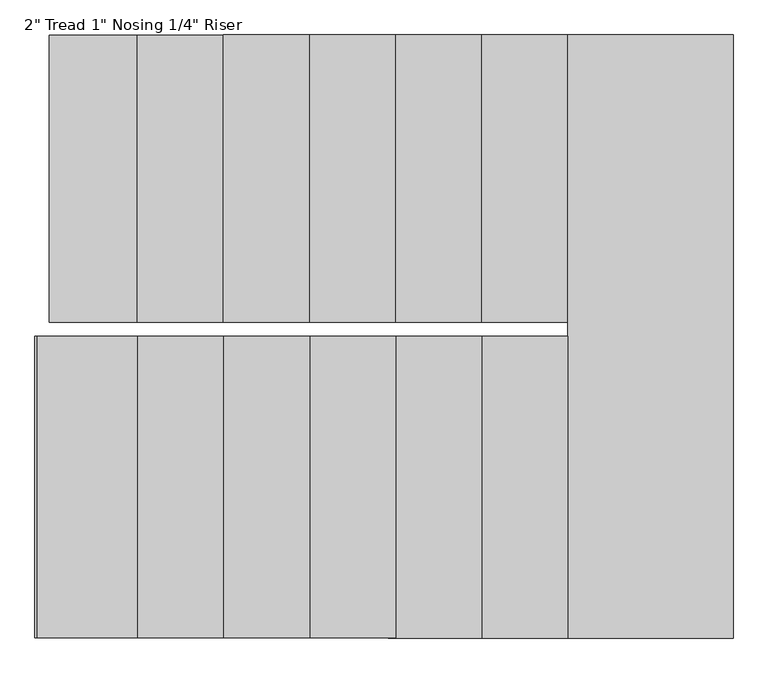
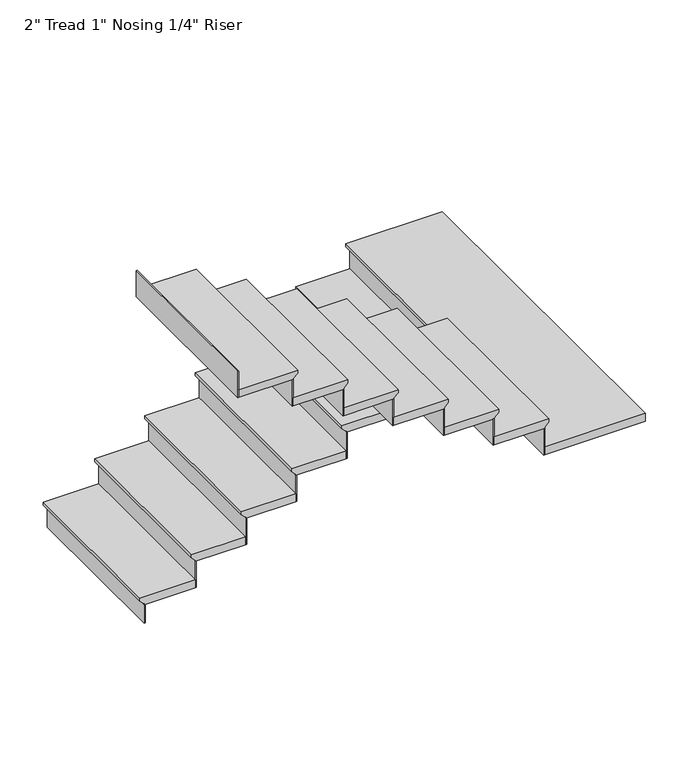
"""IFC4 building model written with IfcOpenShell, lengths in millimetres: stair flight geometry."""

from ifc_helpers import new_model, si_unit, origin, place, context, project, spatial, faceted_brep, source, transform, mapped, element, save


def stair_flight_57dbdc02(model_context):
    return source(origin(), model_context, "Body", "Brep", [
        faceted_brep([(-1167.6638307, -167.7482799, 12951.8833333), (-1167.6638307, -167.7482799, 12970.9333333), (-1167.6638307, 848.2517201, 12970.9333333), (-1167.6638307, 848.2517201, 12951.8833333), (-1142.2638307, -167.7482799, 12926.4833333), (-1142.2638307, 848.2517201, 12926.4833333), (-831.1138307, -167.7482799, 12970.9333333), (-831.1138307, 848.2517201, 12970.9333333), (-1142.2638307, 848.2517201, 12920.1333333), (-831.1138307, 848.2517201, 12920.1333333), (-831.1138307, -167.7482799, 12920.1333333), (-1142.2638307, -167.7482799, 12920.1333333)], [[[0, 1, 2, 3]], [[4, 0, 3, 5]], [[2, 1, 6, 7]], [[8, 9, 10, 11]], [[2, 7, 9, 8, 5, 3]], [[8, 11, 4, 5]], [[6, 1, 0, 4, 11, 10]], [[7, 6, 10, 9]]]),
        faceted_brep([(-1142.2638307, -167.7482799, 12920.1333333), (-1142.2638307, -167.7482799, 12801.6), (-1135.9138307, -167.7482799, 12801.6), (-1135.9138307, -167.7482799, 12920.1333333), (-1142.2638307, 848.2517201, 12920.1333333), (-1135.9138307, 848.2517201, 12920.1333333), (-1135.9138307, 848.2517201, 12801.6), (-1142.2638307, 848.2517201, 12801.6)], [[[0, 1, 2, 3]], [[4, 5, 6, 7]], [[1, 0, 4, 7]], [[2, 1, 7, 6]], [[3, 2, 6, 5]], [[0, 3, 5, 4]]]),
        faceted_brep([(-831.1138307, -167.7482799, 13089.4666667), (-831.1138307, -167.7482799, 12920.1333333), (-824.7638307, -167.7482799, 12920.1333333), (-824.7638307, -167.7482799, 13089.4666667), (-831.1138307, 848.2517201, 13089.4666667), (-824.7638307, 848.2517201, 13089.4666667), (-824.7638307, 848.2517201, 12920.1333333), (-831.1138307, 848.2517201, 12920.1333333)], [[[0, 1, 2, 3]], [[4, 5, 6, 7]], [[1, 0, 4, 7]], [[2, 1, 7, 6]], [[3, 2, 6, 5]], [[0, 3, 5, 4]]]),
        faceted_brep([(-856.5138307, 848.2517201, 13140.2666667), (-856.5138307, -167.7482799, 13140.2666667), (-526.3138307, -167.7482799, 13140.2666667), (-526.3138307, 848.2517201, 13140.2666667), (-831.1138307, 848.2517201, 13089.4666667), (-526.3138307, 848.2517201, 13089.4666667), (-526.3138307, -167.7482799, 13089.4666667), (-831.1138307, -167.7482799, 13089.4666667), (-831.1138307, 848.2517201, 13095.8166667), (-856.5138307, 848.2517201, 13121.2166667), (-831.1138307, -167.7482799, 13095.8166667), (-856.5138307, -167.7482799, 13121.2166667)], [[[0, 1, 2, 3]], [[4, 5, 6, 7]], [[0, 3, 5, 4, 8, 9]], [[4, 7, 10, 8]], [[2, 1, 11, 10, 7, 6]], [[3, 2, 6, 5]], [[11, 1, 0, 9]], [[10, 11, 9, 8]]]),
        faceted_brep([(-526.3138307, -167.7482799, 13258.8), (-526.3138307, -167.7482799, 13089.4666667), (-519.9638307, -167.7482799, 13089.4666667), (-519.9638307, -167.7482799, 13258.8), (-526.3138307, 848.2517201, 13258.8), (-519.9638307, 848.2517201, 13258.8), (-519.9638307, 848.2517201, 13089.4666667), (-526.3138307, 848.2517201, 13089.4666667)], [[[0, 1, 2, 3]], [[4, 5, 6, 7]], [[1, 0, 4, 7]], [[2, 1, 7, 6]], [[3, 2, 6, 5]], [[0, 3, 5, 4]]]),
        faceted_brep([(-551.7138307, 848.2517201, 13309.6), (-551.7138307, -167.7482799, 13309.6), (-221.5138307, -167.7482799, 13309.6), (-221.5138307, 848.2517201, 13309.6), (-526.3138307, 848.2517201, 13258.8), (-221.5138307, 848.2517201, 13258.8), (-221.5138307, -167.7482799, 13258.8), (-526.3138307, -167.7482799, 13258.8), (-526.3138307, 848.2517201, 13265.15), (-551.7138307, 848.2517201, 13290.55), (-526.3138307, -167.7482799, 13265.15), (-551.7138307, -167.7482799, 13290.55)], [[[0, 1, 2, 3]], [[4, 5, 6, 7]], [[0, 3, 5, 4, 8, 9]], [[4, 7, 10, 8]], [[2, 1, 11, 10, 7, 6]], [[3, 2, 6, 5]], [[11, 1, 0, 9]], [[10, 11, 9, 8]]]),
        faceted_brep([(-221.5138307, -167.7482799, 13428.1333333), (-221.5138307, -167.7482799, 13258.8), (-215.1638307, -167.7482799, 13258.8), (-215.1638307, -167.7482799, 13428.1333333), (-221.5138307, 848.2517201, 13428.1333333), (-215.1638307, 848.2517201, 13428.1333333), (-215.1638307, 848.2517201, 13258.8), (-221.5138307, 848.2517201, 13258.8)], [[[0, 1, 2, 3]], [[4, 5, 6, 7]], [[1, 0, 4, 7]], [[2, 1, 7, 6]], [[3, 2, 6, 5]], [[0, 3, 5, 4]]]),
        faceted_brep([(-246.9138307, 848.2517201, 13478.9333333), (-246.9138307, -167.7482799, 13478.9333333), (83.2861693, -167.7482799, 13478.9333333), (83.2861693, 848.2517201, 13478.9333333), (-221.5138307, 848.2517201, 13428.1333333), (83.2861693, 848.2517201, 13428.1333333), (83.2861693, -167.7482799, 13428.1333333), (-221.5138307, -167.7482799, 13428.1333333), (-221.5138307, 848.2517201, 13434.4833333), (-246.9138307, 848.2517201, 13459.8833333), (-221.5138307, -167.7482799, 13434.4833333), (-246.9138307, -167.7482799, 13459.8833333)], [[[0, 1, 2, 3]], [[4, 5, 6, 7]], [[0, 3, 5, 4, 8, 9]], [[4, 7, 10, 8]], [[2, 1, 11, 10, 7, 6]], [[3, 2, 6, 5]], [[11, 1, 0, 9]], [[10, 11, 9, 8]]]),
        faceted_brep([(83.2861693, -167.7482799, 13597.4666667), (83.2861693, -167.7482799, 13428.1333333), (89.6361693, -167.7482799, 13428.1333333), (89.6361693, -167.7482799, 13597.4666667), (83.2861693, 848.2517201, 13597.4666667), (89.6361693, 848.2517201, 13597.4666667), (89.6361693, 848.2517201, 13428.1333333), (83.2861693, 848.2517201, 13428.1333333)], [[[0, 1, 2, 3]], [[4, 5, 6, 7]], [[1, 0, 4, 7]], [[2, 1, 7, 6]], [[3, 2, 6, 5]], [[0, 3, 5, 4]]]),
        faceted_brep([(57.8861693, 848.2517201, 13648.2666667), (57.8861693, -167.7482799, 13648.2666667), (388.0861693, -167.7482799, 13648.2666667), (388.0861693, 848.2517201, 13648.2666667), (83.2861693, 848.2517201, 13597.4666667), (388.0861693, 848.2517201, 13597.4666667), (388.0861693, -167.7482799, 13597.4666667), (83.2861693, -167.7482799, 13597.4666667), (83.2861693, 848.2517201, 13603.8166667), (57.8861693, 848.2517201, 13629.2166667), (83.2861693, -167.7482799, 13603.8166667), (57.8861693, -167.7482799, 13629.2166667)], [[[0, 1, 2, 3]], [[4, 5, 6, 7]], [[0, 3, 5, 4, 8, 9]], [[4, 7, 10, 8]], [[2, 1, 11, 10, 7, 6]], [[3, 2, 6, 5]], [[11, 1, 0, 9]], [[10, 11, 9, 8]]]),
        faceted_brep([(388.0861693, -167.7482799, 13766.8), (388.0861693, -167.7482799, 13597.4666667), (394.4361693, -167.7482799, 13597.4666667), (394.4361693, -167.7482799, 13766.8), (388.0861693, 848.2517201, 13766.8), (394.4361693, 848.2517201, 13766.8), (394.4361693, 848.2517201, 13597.4666667), (388.0861693, 848.2517201, 13597.4666667)], [[[0, 1, 2, 3]], [[4, 5, 6, 7]], [[1, 0, 4, 7]], [[2, 1, 7, 6]], [[3, 2, 6, 5]], [[0, 3, 5, 4]]]),
        faceted_brep([(362.6861693, 848.2517201, 13817.6), (362.6861693, -167.7482799, 13817.6), (692.8861693, -167.7482799, 13817.6), (692.8861693, 848.2517201, 13817.6), (388.0861693, 848.2517201, 13766.8), (692.8861693, 848.2517201, 13766.8), (692.8861693, -167.7482799, 13766.8), (388.0861693, -167.7482799, 13766.8), (388.0861693, 848.2517201, 13773.15), (362.6861693, 848.2517201, 13798.55), (388.0861693, -167.7482799, 13773.15), (362.6861693, -167.7482799, 13798.55)], [[[0, 1, 2, 3]], [[4, 5, 6, 7]], [[0, 3, 5, 4, 8, 9]], [[4, 7, 10, 8]], [[2, 1, 11, 10, 7, 6]], [[3, 2, 6, 5]], [[11, 1, 0, 9]], [[10, 11, 9, 8]]]),
        faceted_brep([(692.8861693, -167.7482799, 13936.1333333), (692.8861693, -167.7482799, 13766.8), (699.2361693, -167.7482799, 13766.8), (699.2361693, -167.7482799, 13936.1333333), (692.8861693, 848.2517201, 13936.1333333), (699.2361693, 848.2517201, 13936.1333333), (699.2361693, 848.2517201, 13766.8), (692.8861693, 848.2517201, 13766.8)], [[[0, 1, 2, 3]], [[4, 5, 6, 7]], [[1, 0, 4, 7]], [[2, 1, 7, 6]], [[3, 2, 6, 5]], [[0, 3, 5, 4]]]),
        faceted_brep([(642.0861693, -1285.3482799, 13986.9333333), (1251.6861693, -1285.3482799, 13986.9333333), (1251.6861693, 848.2517201, 13986.9333333), (667.4861693, 848.2517201, 13986.9333333), (667.4861693, -218.5482799, 13986.9333333), (642.0861693, -218.5482799, 13986.9333333), (1251.6861693, -1285.3482799, 13936.1333333), (642.0861693, -1285.3482799, 13936.1333333), (642.0861693, -218.5482799, 13936.1333333), (667.4861693, -218.5482799, 13936.1333333), (667.4861693, -167.7482799, 13936.1333333), (692.8861693, -167.7482799, 13936.1333333), (692.8861693, 848.2517201, 13936.1333333), (1251.6861693, 848.2517201, 13936.1333333), (692.8861693, 848.2517201, 13942.4833333), (667.4861693, 848.2517201, 13967.8833333), (692.8861693, -167.7482799, 13942.4833333), (667.4861693, -167.7482799, 13967.8833333)], [[[0, 1, 2, 3, 4, 5]], [[6, 7, 8, 9, 10, 11, 12, 13]], [[1, 0, 7, 6]], [[2, 1, 6, 13]], [[3, 2, 13, 12, 14, 15]], [[12, 11, 16, 14]], [[11, 10, 17, 16]], [[4, 3, 15, 17, 10, 9]], [[5, 4, 9, 8]], [[0, 5, 8, 7]], [[15, 14, 16, 17]]]),
        faceted_brep([(642.0861693, -218.5482799, 14105.4666667), (642.0861693, -218.5482799, 13936.1333333), (635.7361693, -218.5482799, 13936.1333333), (635.7361693, -218.5482799, 14105.4666667), (642.0861693, -1285.3482799, 14105.4666667), (635.7361693, -1285.3482799, 14105.4666667), (635.7361693, -1285.3482799, 13936.1333333), (642.0861693, -1285.3482799, 13936.1333333)], [[[0, 1, 2, 3]], [[4, 5, 6, 7]], [[1, 0, 4, 7]], [[2, 1, 7, 6]], [[3, 2, 6, 5]], [[0, 3, 5, 4]]]),
        faceted_brep([(667.4861693, -1285.3482799, 14156.2666667), (667.4861693, -218.5482799, 14156.2666667), (337.2861693, -218.5482799, 14156.2666667), (337.2861693, -1285.3482799, 14156.2666667), (642.0861693, -1285.3482799, 14105.4666667), (337.2861693, -1285.3482799, 14105.4666667), (337.2861693, -218.5482799, 14105.4666667), (642.0861693, -218.5482799, 14105.4666667), (642.0861693, -1285.3482799, 14111.8166667), (667.4861693, -1285.3482799, 14137.2166667), (642.0861693, -218.5482799, 14111.8166667), (667.4861693, -218.5482799, 14137.2166667)], [[[0, 1, 2, 3]], [[4, 5, 6, 7]], [[0, 3, 5, 4, 8, 9]], [[4, 7, 10, 8]], [[2, 1, 11, 10, 7, 6]], [[3, 2, 6, 5]], [[11, 1, 0, 9]], [[10, 11, 9, 8]]]),
        faceted_brep([(337.2861693, -218.5482799, 14274.8), (337.2861693, -218.5482799, 14105.4666667), (330.9361693, -218.5482799, 14105.4666667), (330.9361693, -218.5482799, 14274.8), (337.2861693, -1285.3482799, 14274.8), (330.9361693, -1285.3482799, 14274.8), (330.9361693, -1285.3482799, 14105.4666667), (337.2861693, -1285.3482799, 14105.4666667)], [[[0, 1, 2, 3]], [[4, 5, 6, 7]], [[1, 0, 4, 7]], [[2, 1, 7, 6]], [[3, 2, 6, 5]], [[0, 3, 5, 4]]]),
        faceted_brep([(362.6861693, -1285.3482799, 14325.6), (362.6861693, -218.5482799, 14325.6), (32.4861693, -218.5482799, 14325.6), (32.4861693, -1285.3482799, 14325.6), (337.2861693, -1285.3482799, 14274.8), (32.4861693, -1285.3482799, 14274.8), (32.4861693, -218.5482799, 14274.8), (337.2861693, -218.5482799, 14274.8), (337.2861693, -1285.3482799, 14281.15), (362.6861693, -1285.3482799, 14306.55), (337.2861693, -218.5482799, 14281.15), (362.6861693, -218.5482799, 14306.55)], [[[0, 1, 2, 3]], [[4, 5, 6, 7]], [[0, 3, 5, 4, 8, 9]], [[4, 7, 10, 8]], [[2, 1, 11, 10, 7, 6]], [[3, 2, 6, 5]], [[11, 1, 0, 9]], [[10, 11, 9, 8]]]),
        faceted_brep([(32.4861693, -218.5482799, 14444.1333333), (32.4861693, -218.5482799, 14274.8), (26.1361693, -218.5482799, 14274.8), (26.1361693, -218.5482799, 14444.1333333), (32.4861693, -1285.3482799, 14444.1333333), (26.1361693, -1285.3482799, 14444.1333333), (26.1361693, -1285.3482799, 14274.8), (32.4861693, -1285.3482799, 14274.8)], [[[0, 1, 2, 3]], [[4, 5, 6, 7]], [[1, 0, 4, 7]], [[2, 1, 7, 6]], [[3, 2, 6, 5]], [[0, 3, 5, 4]]]),
        faceted_brep([(57.8861693, -1285.3482799, 14494.9333333), (57.8861693, -218.5482799, 14494.9333333), (-272.3138307, -218.5482799, 14494.9333333), (-272.3138307, -1285.3482799, 14494.9333333), (32.4861693, -1285.3482799, 14444.1333333), (-272.3138307, -1285.3482799, 14444.1333333), (-272.3138307, -218.5482799, 14444.1333333), (32.4861693, -218.5482799, 14444.1333333), (32.4861693, -1285.3482799, 14450.4833333), (57.8861693, -1285.3482799, 14475.8833333), (32.4861693, -218.5482799, 14450.4833333), (57.8861693, -218.5482799, 14475.8833333)], [[[0, 1, 2, 3]], [[4, 5, 6, 7]], [[0, 3, 5, 4, 8, 9]], [[4, 7, 10, 8]], [[2, 1, 11, 10, 7, 6]], [[3, 2, 6, 5]], [[11, 1, 0, 9]], [[10, 11, 9, 8]]]),
        faceted_brep([(-272.3138307, -218.5482799, 14613.4666667), (-272.3138307, -218.5482799, 14444.1333333), (-278.6638307, -218.5482799, 14444.1333333), (-278.6638307, -218.5482799, 14613.4666667), (-272.3138307, -1285.3482799, 14613.4666667), (-278.6638307, -1285.3482799, 14613.4666667), (-278.6638307, -1285.3482799, 14444.1333333), (-272.3138307, -1285.3482799, 14444.1333333)], [[[0, 1, 2, 3]], [[4, 5, 6, 7]], [[1, 0, 4, 7]], [[2, 1, 7, 6]], [[3, 2, 6, 5]], [[0, 3, 5, 4]]]),
        faceted_brep([(-246.9138307, -1285.3482799, 14664.2666667), (-246.9138307, -218.5482799, 14664.2666667), (-577.1138307, -218.5482799, 14664.2666667), (-577.1138307, -1285.3482799, 14664.2666667), (-272.3138307, -1285.3482799, 14613.4666667), (-577.1138307, -1285.3482799, 14613.4666667), (-577.1138307, -218.5482799, 14613.4666667), (-272.3138307, -218.5482799, 14613.4666667), (-272.3138307, -1285.3482799, 14619.8166667), (-246.9138307, -1285.3482799, 14645.2166667), (-272.3138307, -218.5482799, 14619.8166667), (-246.9138307, -218.5482799, 14645.2166667)], [[[0, 1, 2, 3]], [[4, 5, 6, 7]], [[0, 3, 5, 4, 8, 9]], [[4, 7, 10, 8]], [[2, 1, 11, 10, 7, 6]], [[3, 2, 6, 5]], [[11, 1, 0, 9]], [[10, 11, 9, 8]]]),
        faceted_brep([(-577.1138307, -218.5482799, 14782.8), (-577.1138307, -218.5482799, 14613.4666667), (-583.4638307, -218.5482799, 14613.4666667), (-583.4638307, -218.5482799, 14782.8), (-577.1138307, -1285.3482799, 14782.8), (-583.4638307, -1285.3482799, 14782.8), (-583.4638307, -1285.3482799, 14613.4666667), (-577.1138307, -1285.3482799, 14613.4666667)], [[[0, 1, 2, 3]], [[4, 5, 6, 7]], [[1, 0, 4, 7]], [[2, 1, 7, 6]], [[3, 2, 6, 5]], [[0, 3, 5, 4]]]),
        faceted_brep([(-551.7138307, -1285.3482799, 14833.6), (-551.7138307, -218.5482799, 14833.6), (-881.9138307, -218.5482799, 14833.6), (-881.9138307, -1285.3482799, 14833.6), (-577.1138307, -1285.3482799, 14782.8), (-881.9138307, -1285.3482799, 14782.8), (-881.9138307, -218.5482799, 14782.8), (-577.1138307, -218.5482799, 14782.8), (-577.1138307, -1285.3482799, 14789.15), (-551.7138307, -1285.3482799, 14814.55), (-577.1138307, -218.5482799, 14789.15), (-551.7138307, -218.5482799, 14814.55)], [[[0, 1, 2, 3]], [[4, 5, 6, 7]], [[0, 3, 5, 4, 8, 9]], [[4, 7, 10, 8]], [[2, 1, 11, 10, 7, 6]], [[3, 2, 6, 5]], [[11, 1, 0, 9]], [[10, 11, 9, 8]]]),
        faceted_brep([(-881.9138307, -218.5482799, 14952.1333333), (-881.9138307, -218.5482799, 14782.8), (-888.2638307, -218.5482799, 14782.8), (-888.2638307, -218.5482799, 14952.1333333), (-881.9138307, -1285.3482799, 14952.1333333), (-888.2638307, -1285.3482799, 14952.1333333), (-888.2638307, -1285.3482799, 14782.8), (-881.9138307, -1285.3482799, 14782.8)], [[[0, 1, 2, 3]], [[4, 5, 6, 7]], [[1, 0, 4, 7]], [[2, 1, 7, 6]], [[3, 2, 6, 5]], [[0, 3, 5, 4]]]),
        faceted_brep([(-1212.1138307, -218.5482799, 15121.4666667), (-1212.1138307, -218.5482799, 14952.1333333), (-1218.4638307, -218.5482799, 14952.1333333), (-1218.4638307, -218.5482799, 15121.4666667), (-1212.1138307, -1285.3482799, 15121.4666667), (-1218.4638307, -1285.3482799, 15121.4666667), (-1218.4638307, -1285.3482799, 14952.1333333), (-1212.1138307, -1285.3482799, 14952.1333333)], [[[0, 1, 2, 3]], [[4, 5, 6, 7]], [[1, 0, 4, 7]], [[2, 1, 7, 6]], [[3, 2, 6, 5]], [[0, 3, 5, 4]]]),
        faceted_brep([(-856.5138307, -1285.3482799, 15002.9333333), (-856.5138307, -218.5482799, 15002.9333333), (-1212.1138307, -218.5482799, 15002.9333333), (-1212.1138307, -1285.3482799, 15002.9333333), (-881.9138307, -1285.3482799, 14952.1333333), (-1212.1138307, -1285.3482799, 14952.1333333), (-1212.1138307, -218.5482799, 14952.1333333), (-881.9138307, -218.5482799, 14952.1333333), (-881.9138307, -1285.3482799, 14958.4833333), (-856.5138307, -1285.3482799, 14983.8833333), (-881.9138307, -218.5482799, 14958.4833333), (-856.5138307, -218.5482799, 14983.8833333)], [[[0, 1, 2, 3]], [[4, 5, 6, 7]], [[0, 3, 5, 4, 8, 9]], [[4, 7, 10, 8]], [[2, 1, 11, 10, 7, 6]], [[3, 2, 6, 5]], [[11, 1, 0, 9]], [[10, 11, 9, 8]]]),
    ])


if __name__ == "__main__":
    model = new_model("IFC4")
    model_context = context("Model", 3, world=origin())
    ifc_project = project(units=[si_unit("LENGTHUNIT", "METRE", prefix="MILLI")], contexts=[model_context])
    site = spatial("IfcSite", under=ifc_project)
    building = spatial("IfcBuilding", under=site)
    placement = place(None, origin())
    stair_flight_shape = stair_flight_57dbdc02(model_context)
    element("IfcStairFlight", 1, ObjectType="2\" Tread 1\" Nosing 1/4\" Riser", at=placement, inside=building, context=model_context, shape_type="MappedRepresentation", body=[
        mapped(stair_flight_shape, transform((0.0, 0.0, 0.0), x_axis=(1.0, 0.0, 0.0), y_axis=(0.0, 1.0, 0.0), z_axis=(0.0, 0.0, 1.0))),
    ])
    save(model, "model.ifc")
